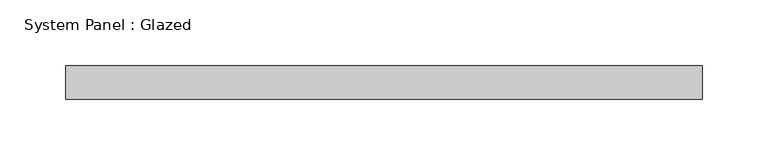
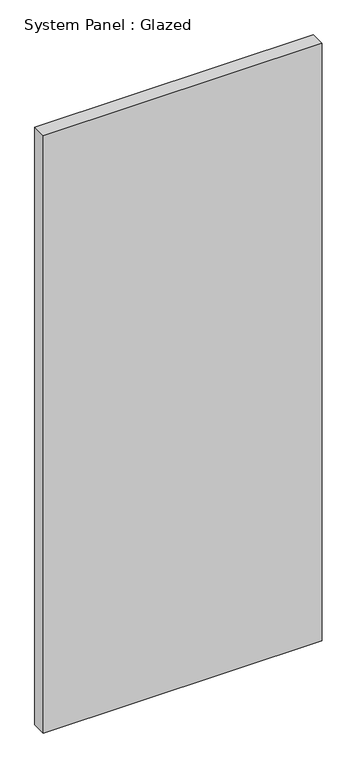
"""IFC4 building model written with IfcOpenShell, lengths in millimetres: plate geometry, System Panel : Glazed."""

from ifc_helpers import new_model, si_unit, origin, origin_with_axes, place, context, project, spatial, polyline, outline, extrude, source, transform, mapped, element, save


def system_panel_glazed_1bcf12e0(model_context):
    return source(origin(), model_context, "Body", "SweptSolid", [
        extrude(outline(polyline([(241.3, 19.05), (-241.3, 19.05), (-241.3, 44.45), (241.3, 44.45), (241.3, 19.05)])), origin_with_axes(), (0.0, 0.0, 1.0), 1092.2),
    ])


if __name__ == "__main__":
    model = new_model("IFC4")
    model_context = context("Model", 3, world=origin())
    ifc_project = project(units=[si_unit("LENGTHUNIT", "METRE", prefix="MILLI")], contexts=[model_context])
    site = spatial("IfcSite", under=ifc_project)
    building = spatial("IfcBuilding", under=site)
    placement = place(None, origin())
    system_panel_glazed_shape = system_panel_glazed_1bcf12e0(model_context)
    element("IfcPlate", 1, ObjectType="System Panel : Glazed", at=placement, inside=building, context=model_context, shape_type="MappedRepresentation", body=[
        mapped(system_panel_glazed_shape, transform((0.0, 0.0, 0.0), x_axis=(1.0, 0.0, 0.0), y_axis=(0.0, 1.0, 0.0), z_axis=(0.0, 0.0, 1.0))),
    ])
    save(model, "model.ifc")

# Revit data of these elements
# Type "System Panel : Glazed"
#   Construction Type Id = "GSP4R"
#   Analytic Construction = "1/8 in Pilkington single glazing"
#   Visual Light Transmittance = 0.9
#   Solar Heat Gain Coefficient = 0.86
#   Heat Transfer Coefficient (U) = 1.18115 BTU/(h·ft²·°F)
#   Define Thermal Properties by = 1
# Element 1 (IfcPlate, "System Panel : Glazed")
#   Materials on its faces: "Glass"
# Materials
#   "Glass": class "Glass", colour RGB 0 128 192, transparency 0.75, Description = "Soda Lime Glass", Cost = 0
